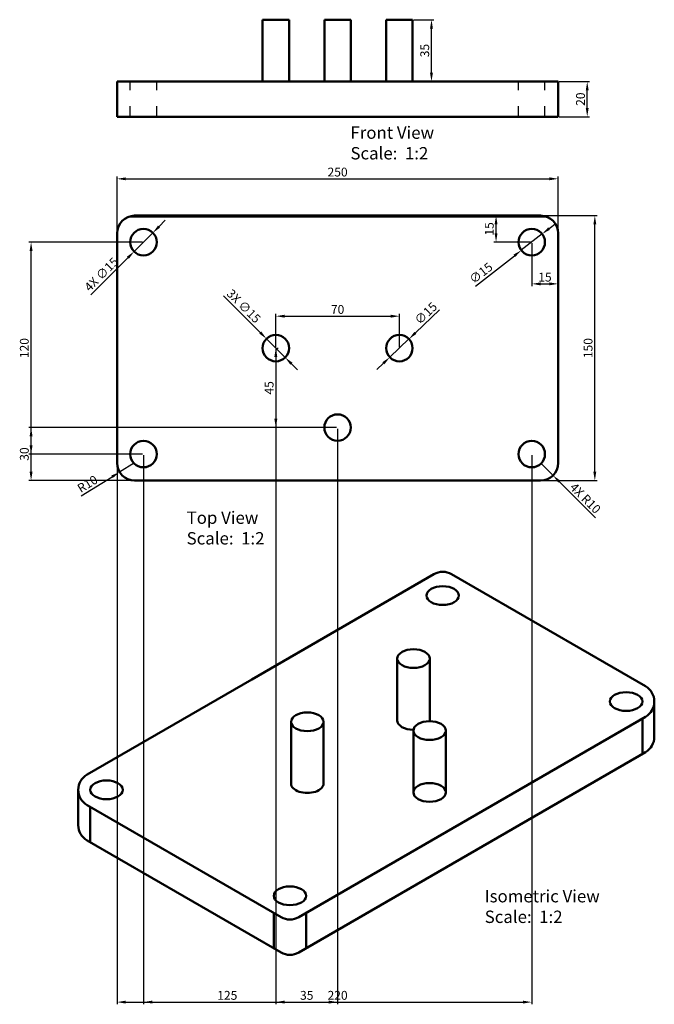
# Model space of a CAD drawing. Units: millimetres. Extents: x 2577 to 3382, y -259 to 299.
# Tile 1 of 2: x 2577 to 2937, y -259 to 299. Entities that reach past the tile are written whole.
import ezdxf

# ---------------------------------------------------------------- set-up
doc = ezdxf.new("R2010")
doc.units = ezdxf.units.MM
doc.linetypes.add('ACAD_ISO03W100', pattern=[30, 12, -18])
for name, color, linetype, lineweight in [('M-DIMS', 2, 'Continuous', 25), ('M-HIDN', 7, 'ACAD_ISO03W100', 25), ('M-OUTL', 7, 'Continuous', 50), ('M-TEXT', 7, 'Continuous', 25)]:
    doc.layers.add(name, color=color, linetype=linetype, lineweight=lineweight)
doc.styles.get("Standard").update_dxf_attribs({"font": 'arial.ttf'})
doc.dimstyles.new('ISO-25', dxfattribs={"dimtxt": 5, "dimasz": 5, "dimexe": 1.25, "dimexo": 0.625, "dimtad": 1, "dimdec": 0, "dimtxsty": 'Standard', "dimcen": 2.5, "dimadec": 0, "dimazin": 0, "dimtfac": 1, "dimtdec": 0, "dimtmove": 0, "dimatfit": 3, "dimfxl": 1, "dimarcsym": 0})

# ---------------------------------------------------------------- blocks, each defined once
blk = doc.blocks.new('*D1')
at = {"layer": 'Defpoints', "color": 0, "transparency": 16777216}
for p in [(2792.35, 130.65), (2722.35, 112.58), (2792.35, 112.58)]:
    blk.add_point(p, dxfattribs=at)
at = {"layer": 'M-DIMS', "color": 0, "lineweight": -2, "transparency": 16777216}
for p, q in [((2722.35, 113.2), (2722.35, 131.9)), ((2727.35, 130.65), (2787.35, 130.65)), ((2792.35, 113.2), (2792.35, 131.9))]:
    blk.add_line(p, q, dxfattribs=at)
at = {"layer": 'M-DIMS', "color": 0, "transparency": 16777216}
for points in [[(2727.35, 131.49), (2727.35, 129.82), (2722.35, 130.65)], [(2787.35, 131.49), (2787.35, 129.82), (2792.35, 130.65)]]:
    blk.add_solid(points, dxfattribs=at)
at = {"layer": 'M-DIMS', "color": 0, "transparency": 16777216, "insert": (2757.35, 133.83), "char_height": 5, "attachment_point": 5}
blk.add_mtext('70', dxfattribs=at)
blk = doc.blocks.new('*D2')
at = {"layer": 'Defpoints', "color": 0, "transparency": 16777216}
for p in [(2722.35, 112.58), (2722.35, 67.58), (2757.35, 67.58)]:
    blk.add_point(p, dxfattribs=at)
at = {"layer": 'M-DIMS', "color": 0, "lineweight": -2, "transparency": 16777216}
for p, q in [((2722.97, 112.58), (2723.6, 112.58)), ((2722.35, 107.58), (2722.35, 72.58)), ((2756.72, 67.58), (2721.1, 67.58))]:
    blk.add_line(p, q, dxfattribs=at)
at = {"layer": 'M-DIMS', "color": 0, "transparency": 16777216}
for points in [[(2721.52, 107.58), (2723.18, 107.58), (2722.35, 112.58)], [(2721.52, 72.58), (2723.18, 72.58), (2722.35, 67.58)]]:
    blk.add_solid(points, dxfattribs=at)
at = {"layer": 'M-DIMS', "color": 0, "transparency": 16777216, "insert": (2719.18, 90.08), "char_height": 5, "attachment_point": 5, "rotation": 90}
blk.add_mtext('45', dxfattribs=at)
blk = doc.blocks.new('*D3')
at = {"layer": 'Defpoints', "color": 0, "transparency": 16777216}
for p in [(2882.35, 208.44), (2632.35, 177.58), (2882.35, 177.58)]:
    blk.add_point(p, dxfattribs=at)
at = {"layer": 'M-DIMS', "color": 0, "lineweight": -2, "transparency": 16777216}
for p, q in [((2632.35, 178.2), (2632.35, 209.69)), ((2637.35, 208.44), (2877.35, 208.44)), ((2882.35, 178.2), (2882.35, 209.69))]:
    blk.add_line(p, q, dxfattribs=at)
at = {"layer": 'M-DIMS', "color": 0, "transparency": 16777216}
for points in [[(2637.35, 209.27), (2637.35, 207.61), (2632.35, 208.44)], [(2877.35, 209.27), (2877.35, 207.61), (2882.35, 208.44)]]:
    blk.add_solid(points, dxfattribs=at)
at = {"layer": 'M-DIMS', "color": 0, "transparency": 16777216, "insert": (2757.35, 211.62), "char_height": 5, "attachment_point": 5}
blk.add_mtext('250', dxfattribs=at)
blk = doc.blocks.new('*D4')
at = {"layer": 'Defpoints', "color": 0, "transparency": 16777216}
for p in [(2872.35, 187.58), (2903.11, 187.58), (2872.35, 37.58)]:
    blk.add_point(p, dxfattribs=at)
at = {"layer": 'M-DIMS', "color": 0, "lineweight": -2, "transparency": 16777216}
for p, q in [((2872.97, 187.58), (2904.36, 187.58)), ((2903.11, 42.58), (2903.11, 182.58)), ((2872.97, 37.58), (2904.36, 37.58))]:
    blk.add_line(p, q, dxfattribs=at)
at = {"layer": 'M-DIMS', "color": 0, "transparency": 16777216}
for points in [[(2902.28, 182.58), (2903.94, 182.58), (2903.11, 187.58)], [(2902.28, 42.58), (2903.94, 42.58), (2903.11, 37.58)]]:
    blk.add_solid(points, dxfattribs=at)
at = {"layer": 'M-DIMS', "color": 0, "transparency": 16777216, "insert": (2899.93, 112.58), "char_height": 5, "attachment_point": 5, "rotation": 90}
blk.add_mtext('150', dxfattribs=at)
blk = doc.blocks.new('*D5')
at = {"layer": 'Defpoints', "color": 0, "transparency": 16777216}
for p in [(2847.14, 187.58), (2867.35, 187.58), (2867.35, 172.58)]:
    blk.add_point(p, dxfattribs=at)
at = {"layer": 'M-DIMS', "color": 0, "lineweight": -2, "transparency": 16777216}
for p, q in [((2866.72, 187.58), (2845.89, 187.58)), ((2847.14, 177.58), (2847.14, 182.58)), ((2866.72, 172.58), (2845.89, 172.58))]:
    blk.add_line(p, q, dxfattribs=at)
at = {"layer": 'M-DIMS', "color": 0, "transparency": 16777216}
for points in [[(2846.31, 182.58), (2847.97, 182.58), (2847.14, 187.58)], [(2846.31, 177.58), (2847.97, 177.58), (2847.14, 172.58)]]:
    blk.add_solid(points, dxfattribs=at)
at = {"layer": 'M-DIMS', "color": 0, "transparency": 16777216, "insert": (2843.96, 180.08), "char_height": 5, "attachment_point": 5, "rotation": 90}
blk.add_mtext('15', dxfattribs=at)
blk = doc.blocks.new('*D6')
at = {"layer": 'Defpoints', "color": 0, "transparency": 16777216}
for p in [(2867.35, 172.58), (2882.35, 172.58), (2882.35, 148.96)]:
    blk.add_point(p, dxfattribs=at)
at = {"layer": 'M-DIMS', "color": 0, "lineweight": -2, "transparency": 16777216}
for p, q in [((2867.35, 171.95), (2867.35, 147.71)), ((2882.35, 171.95), (2882.35, 147.71)), ((2872.35, 148.96), (2877.35, 148.96))]:
    blk.add_line(p, q, dxfattribs=at)
at = {"layer": 'M-DIMS', "color": 0, "transparency": 16777216}
for points in [[(2872.35, 149.79), (2872.35, 148.12), (2867.35, 148.96)], [(2877.35, 149.79), (2877.35, 148.12), (2882.35, 148.96)]]:
    blk.add_solid(points, dxfattribs=at)
at = {"layer": 'M-DIMS', "color": 0, "transparency": 16777216, "insert": (2874.85, 152.13), "char_height": 5, "attachment_point": 5}
blk.add_mtext('15', dxfattribs=at)
blk = doc.blocks.new('*D7')
at = {"layer": 'Defpoints', "color": 0, "transparency": 16777216}
for p in [(2642.35, 47.58), (2633.82, 42.35)]:
    blk.add_point(p, dxfattribs=at)
at = {"layer": 'M-DIMS', "color": 0, "lineweight": -2, "transparency": 16777216}
for p, q in [((2642.35, 47.58), (2633.82, 42.35)), ((2612.01, 28.97), (2629.56, 39.73))]:
    blk.add_line(p, q, dxfattribs=at)
at = {"layer": 'M-DIMS', "color": 0, "transparency": 16777216}
blk.add_solid([(2629.13, 40.44), (2630, 39.02), (2633.82, 42.35)], dxfattribs=at)
at = {"layer": 'M-DIMS', "color": 0, "transparency": 16777216, "insert": (2615.96, 35.12), "char_height": 5, "attachment_point": 5, "rotation": 31.518}
blk.add_mtext('R10', dxfattribs=at)
blk = doc.blocks.new('*D8')
at = {"layer": 'Defpoints', "color": 0, "transparency": 16777216}
for p in [(2797.79, 117.74), (2786.91, 107.41)]:
    blk.add_point(p, dxfattribs=at)
at = {"layer": 'M-DIMS', "color": 0, "lineweight": -2, "transparency": 16777216}
for p, q in [((2815.1, 134.2), (2801.41, 121.19)), ((2786.91, 107.41), (2797.79, 117.74)), ((2783.29, 103.96), (2779.67, 100.52))]:
    blk.add_line(p, q, dxfattribs=at)
at = {"layer": 'M-DIMS', "color": 0, "transparency": 16777216}
for points in [[(2800.84, 121.79), (2801.98, 120.58), (2797.79, 117.74)], [(2782.72, 104.57), (2783.86, 103.36), (2786.91, 107.41)]]:
    blk.add_solid(points, dxfattribs=at)
at = {"layer": 'M-DIMS', "color": 0, "transparency": 16777216, "insert": (2807.78, 131.82), "char_height": 5, "attachment_point": 5, "rotation": 43.5491}
blk.add_mtext('∅15', dxfattribs=at)
blk = doc.blocks.new('*D9')
at = {"layer": 'Defpoints', "color": 0, "transparency": 16777216}
for p in [(2873.26, 177.2), (2861.44, 167.95)]:
    blk.add_point(p, dxfattribs=at)
at = {"layer": 'M-DIMS', "color": 0, "lineweight": -2, "transparency": 16777216}
for p, q in [((2877.19, 180.28), (2881.13, 183.36)), ((2873.26, 177.2), (2861.44, 167.95)), ((2835.55, 147.69), (2857.5, 164.87))]:
    blk.add_line(p, q, dxfattribs=at)
at = {"layer": 'M-DIMS', "color": 0, "transparency": 16777216}
for points in [[(2876.68, 180.93), (2877.71, 179.62), (2873.26, 177.2)], [(2856.99, 165.53), (2858.02, 164.22), (2861.44, 167.95)]]:
    blk.add_solid(points, dxfattribs=at)
at = {"layer": 'M-DIMS', "color": 0, "transparency": 16777216, "insert": (2838.97, 154.58), "char_height": 5, "attachment_point": 5, "rotation": 38.04}
blk.add_mtext('∅15', dxfattribs=at)
blk = doc.blocks.new('*D10')
at = {"layer": 'Defpoints', "color": 0, "transparency": 16777216}
for p in [(2799.85, 298.55), (2810.55, 298.55), (2799.85, 263.55)]:
    blk.add_point(p, dxfattribs=at)
at = {"layer": 'M-DIMS', "color": 0, "lineweight": -2, "transparency": 16777216}
for p, q in [((2800.47, 298.55), (2811.8, 298.55)), ((2810.55, 268.55), (2810.55, 293.55)), ((2800.47, 263.55), (2811.8, 263.55))]:
    blk.add_line(p, q, dxfattribs=at)
at = {"layer": 'M-DIMS', "color": 0, "transparency": 16777216}
for points in [[(2809.71, 293.55), (2811.38, 293.55), (2810.55, 298.55)], [(2809.71, 268.55), (2811.38, 268.55), (2810.55, 263.55)]]:
    blk.add_solid(points, dxfattribs=at)
at = {"layer": 'M-DIMS', "color": 0, "transparency": 16777216, "insert": (2807.37, 281.05), "char_height": 5, "attachment_point": 5, "rotation": 90}
blk.add_mtext('35', dxfattribs=at)
blk = doc.blocks.new('*D11')
at = {"layer": 'Defpoints', "color": 0, "transparency": 16777216}
for p in [(2882.35, 263.55), (2898.8, 263.55), (2882.35, 243.55)]:
    blk.add_point(p, dxfattribs=at)
at = {"layer": 'M-DIMS', "color": 0, "lineweight": -2, "transparency": 16777216}
for p, q in [((2882.97, 263.55), (2900.05, 263.55)), ((2898.8, 248.55), (2898.8, 258.55)), ((2882.97, 243.55), (2900.05, 243.55))]:
    blk.add_line(p, q, dxfattribs=at)
at = {"layer": 'M-DIMS', "color": 0, "transparency": 16777216}
for points in [[(2897.97, 258.55), (2899.63, 258.55), (2898.8, 263.55)], [(2897.97, 248.55), (2899.63, 248.55), (2898.8, 243.55)]]:
    blk.add_solid(points, dxfattribs=at)
at = {"layer": 'M-DIMS', "color": 0, "transparency": 16777216, "insert": (2895.62, 253.55), "char_height": 5, "attachment_point": 5, "rotation": 90}
blk.add_mtext('20', dxfattribs=at)
blk = doc.blocks.new('PIN-D15-H35-FRONT')
for p, q in [((-7.5, 35), (-7.5, 0)), ((7.5, 35), (-7.5, 35)), ((7.5, 35), (7.5, 0))]:
    blk.add_line(p, q)
blk = doc.blocks.new('PIN-D15-H35-ISO')
for p, q in [((-9.19, 0), (-9.19, 35)), ((9.19, 0), (9.19, 35))]:
    blk.add_line(p, q)
blk.add_ellipse((0, 35), major_axis=(-9.19, 0), ratio=0.57735)
blk = doc.blocks.new('BORE-D15-T20-FRONT')
at = {"ltscale": 0.5}
for p, q in [((-7.5, 0), (-7.5, 20)), ((7.5, 0), (7.5, 20))]:
    blk.add_line(p, q, dxfattribs=at)
blk = doc.blocks.new('BORE-D15-TOP')
blk.add_circle((0, 0), 7.5)
blk = doc.blocks.new('BORE-D15-ISO')
blk.add_ellipse((0, 0), major_axis=(-9.19, 0), ratio=0.57735)
blk = doc.blocks.new('PIN-D15-TOP')
blk.add_circle((0, 0), 7.5)
blk = doc.blocks.new('*D25')
at = {"layer": 'Defpoints', "color": 0, "transparency": 16777216}
for p in [(2757.35, 67.58), (2632.35, 47.58), (2757.35, -257.75)]:
    blk.add_point(p, dxfattribs=at)
at = {"layer": 'M-DIMS', "color": 0, "lineweight": -2, "transparency": 16777216}
for p, q in [((2757.35, 66.95), (2757.35, -259)), ((2632.35, 46.95), (2632.35, -259)), ((2637.35, -257.75), (2752.35, -257.75))]:
    blk.add_line(p, q, dxfattribs=at)
at = {"layer": 'M-DIMS', "color": 0, "transparency": 16777216}
for points in [[(2637.35, -256.92), (2637.35, -258.58), (2632.35, -257.75)], [(2752.35, -256.92), (2752.35, -258.58), (2757.35, -257.75)]]:
    blk.add_solid(points, dxfattribs=at)
at = {"layer": 'M-DIMS', "color": 0, "transparency": 16777216, "insert": (2694.85, -254.57), "char_height": 5, "attachment_point": 5}
blk.add_mtext('125', dxfattribs=at)
blk = doc.blocks.new('*D26')
at = {"layer": 'Defpoints', "color": 0, "transparency": 16777216}
for p in [(2583.66, 67.58), (2757.35, 67.58), (2642.35, 37.58)]:
    blk.add_point(p, dxfattribs=at)
at = {"layer": 'M-DIMS', "color": 0, "lineweight": -2, "transparency": 16777216}
for p, q in [((2756.72, 67.58), (2582.41, 67.58)), ((2583.66, 42.58), (2583.66, 62.58)), ((2641.72, 37.58), (2582.41, 37.58))]:
    blk.add_line(p, q, dxfattribs=at)
at = {"layer": 'M-DIMS', "color": 0, "transparency": 16777216}
for points in [[(2582.83, 62.58), (2584.5, 62.58), (2583.66, 67.58)], [(2582.83, 42.58), (2584.5, 42.58), (2583.66, 37.58)]]:
    blk.add_solid(points, dxfattribs=at)
at = {"layer": 'M-DIMS', "color": 0, "transparency": 16777216, "insert": (2580.48, 52.58), "char_height": 5, "attachment_point": 5, "rotation": 90}
blk.add_mtext('30', dxfattribs=at)
blk = doc.blocks.new('*D27')
at = {"layer": 'Defpoints', "color": 0, "transparency": 16777216}
for p in [(2722.35, 112.58), (2757.35, 67.58), (2757.35, -257.75)]:
    blk.add_point(p, dxfattribs=at)
at = {"layer": 'M-DIMS', "color": 0, "lineweight": -2, "transparency": 16777216}
for p, q in [((2722.35, 111.95), (2722.35, -259)), ((2757.35, 66.95), (2757.35, -259)), ((2727.35, -257.75), (2752.35, -257.75))]:
    blk.add_line(p, q, dxfattribs=at)
at = {"layer": 'M-DIMS', "color": 0, "transparency": 16777216}
for points in [[(2727.35, -256.92), (2727.35, -258.58), (2722.35, -257.75)], [(2752.35, -256.92), (2752.35, -258.58), (2757.35, -257.75)]]:
    blk.add_solid(points, dxfattribs=at)
at = {"layer": 'M-DIMS', "color": 0, "transparency": 16777216, "insert": (2739.85, -254.57), "char_height": 5, "attachment_point": 5}
blk.add_mtext('35', dxfattribs=at)
blk = doc.blocks.new('*D36')
at = {"layer": 'Defpoints', "color": 0, "transparency": 16777216}
for p in [(2647.35, 52.58), (2867.35, 52.58), (2867.35, -257.75)]:
    blk.add_point(p, dxfattribs=at)
at = {"layer": 'M-DIMS', "color": 0, "lineweight": -2, "transparency": 16777216}
for p, q in [((2647.35, 51.95), (2647.35, -259)), ((2867.35, 51.95), (2867.35, -259)), ((2652.35, -257.75), (2862.35, -257.75))]:
    blk.add_line(p, q, dxfattribs=at)
at = {"layer": 'M-DIMS', "color": 0, "transparency": 16777216}
for points in [[(2652.35, -256.92), (2652.35, -258.58), (2647.35, -257.75)], [(2862.35, -256.92), (2862.35, -258.58), (2867.35, -257.75)]]:
    blk.add_solid(points, dxfattribs=at)
at = {"layer": 'M-DIMS', "color": 0, "transparency": 16777216, "insert": (2757.35, -254.57), "char_height": 5, "attachment_point": 5}
blk.add_mtext('220', dxfattribs=at)
blk = doc.blocks.new('*D37')
at = {"layer": 'Defpoints', "color": 0, "transparency": 16777216}
for p in [(2583.66, 172.58), (2647.35, 172.58), (2647.35, 52.58)]:
    blk.add_point(p, dxfattribs=at)
at = {"layer": 'M-DIMS', "color": 0, "lineweight": -2, "transparency": 16777216}
for p, q in [((2646.72, 172.58), (2582.41, 172.58)), ((2583.66, 57.58), (2583.66, 167.58)), ((2646.72, 52.58), (2582.41, 52.58))]:
    blk.add_line(p, q, dxfattribs=at)
at = {"layer": 'M-DIMS', "color": 0, "transparency": 16777216}
for points in [[(2582.83, 167.58), (2584.5, 167.58), (2583.66, 172.58)], [(2582.83, 57.58), (2584.5, 57.58), (2583.66, 52.58)]]:
    blk.add_solid(points, dxfattribs=at)
at = {"layer": 'M-DIMS', "color": 0, "transparency": 16777216, "insert": (2580.48, 112.58), "char_height": 5, "attachment_point": 5, "rotation": 90}
blk.add_mtext('120', dxfattribs=at)
blk = doc.blocks.new('*D38')
at = {"layer": 'Defpoints', "color": 0, "transparency": 16777216}
for p in [(2717.05, 117.88), (2727.65, 107.27)]:
    blk.add_point(p, dxfattribs=at)
at = {"layer": 'M-DIMS', "color": 0, "lineweight": -2, "transparency": 16777216}
for p, q in [((2692.76, 142.19), (2713.51, 121.42)), ((2727.65, 107.27), (2717.05, 117.88)), ((2731.18, 103.73), (2734.72, 100.2))]:
    blk.add_line(p, q, dxfattribs=at)
at = {"layer": 'M-DIMS', "color": 0, "transparency": 16777216}
for points in [[(2714.1, 122.01), (2712.93, 120.83), (2717.05, 117.88)], [(2731.77, 104.32), (2730.59, 103.14), (2727.65, 107.27)]]:
    blk.add_solid(points, dxfattribs=at)
at = {"layer": 'M-DIMS', "color": 0, "transparency": 16777216, "insert": (2703.72, 135.92), "char_height": 5, "attachment_point": 5, "rotation": 314.9742}
blk.add_mtext('3X ∅15', dxfattribs=at)
blk = doc.blocks.new('*D39')
at = {"layer": 'Defpoints', "color": 0, "transparency": 16777216}
for p in [(2872.35, 47.58), (2879.42, 40.5)]:
    blk.add_point(p, dxfattribs=at)
at = {"layer": 'M-DIMS', "color": 0, "lineweight": -2, "transparency": 16777216}
for p, q in [((2872.35, 47.58), (2879.42, 40.5)), ((2903.55, 16.38), (2882.96, 36.97))]:
    blk.add_line(p, q, dxfattribs=at)
at = {"layer": 'M-DIMS', "color": 0, "transparency": 16777216}
blk.add_solid([(2883.55, 37.56), (2882.37, 36.38), (2879.42, 40.5)], dxfattribs=at)
at = {"layer": 'M-DIMS', "color": 0, "transparency": 16777216, "insert": (2897.27, 27.15), "char_height": 5, "attachment_point": 5, "rotation": 315.0032}
blk.add_mtext('4X R10', dxfattribs=at)
blk = doc.blocks.new('*D40')
at = {"layer": 'Defpoints', "color": 0, "transparency": 16777216}
for p in [(2652.65, 177.88), (2642.04, 167.27)]:
    blk.add_point(p, dxfattribs=at)
at = {"layer": 'M-DIMS', "color": 0, "lineweight": -2, "transparency": 16777216}
for p, q in [((2656.19, 181.41), (2659.73, 184.95)), ((2652.65, 177.88), (2642.04, 167.27)), ((2617.59, 142.84), (2638.51, 163.74))]:
    blk.add_line(p, q, dxfattribs=at)
at = {"layer": 'M-DIMS', "color": 0, "transparency": 16777216}
for points in [[(2655.6, 182), (2656.78, 180.82), (2652.65, 177.88)], [(2637.92, 164.33), (2639.1, 163.15), (2642.04, 167.27)]]:
    blk.add_solid(points, dxfattribs=at)
at = {"layer": 'M-DIMS', "color": 0, "transparency": 16777216, "insert": (2623.94, 153.87), "char_height": 5, "attachment_point": 5, "rotation": 44.9783}
blk.add_mtext('4X ∅15', dxfattribs=at)

msp = doc.modelspace()

# ---------------------------------------------------------------- linework, layer by layer
at = {"layer": 'M-OUTL'}
for p, q in [((2784.85, 298.55), (2784.85, 263.55)), ((2799.85, 298.55), (2799.85, 263.55)), ((2882.35, 263.55), (2632.35, 263.55)), ((2632.35, 263.55), (2632.35, 243.55)), ((2882.35, 243.55), (2882.35, 263.55)), ((2632.35, 243.55), (2882.35, 243.55)), ((2875.11, 187.19), (2639.59, 187.19)), ((2872.35, 187.58), (2642.35, 187.58)), ((2632.35, 177.58), (2632.35, 47.58)), ((2882.35, 47.58), (2882.35, 177.58)), ((2642.35, 37.58), (2872.35, 37.58)), ((2708.67, -75.05), (2811.92, -15.43)), ((2821.92, -15.43), (2931.82, -78.89)), ((2708.67, -75.05), (2615.41, -128.89)), ((2936.82, -87.55), (2936.82, -107.55)), ((2931.82, -96.21), (2735.32, -209.66)), ((2930.03, -97.24), (2930.03, -117.24)), ((2735.32, -229.66), (2931.82, -116.21)), ((2610.41, -137.55), (2610.41, -157.55)), ((2725.32, -209.66), (2615.41, -146.21)), ((2617.21, -147.24), (2617.21, -167.24)), ((2615.41, -166.21), (2725.32, -229.66)), ((2721.13, -207.24), (2721.13, -227.24)), ((2739.5, -207.24), (2739.5, -227.24))]:
    msp.add_line(p, q, dxfattribs=at)
for centre, start, end in [((2642.35, 177.58), 90, 180), ((2872.35, 177.58), 0, 90), ((2642.35, 47.58), 180, 270), ((2872.35, 47.58), 270, 0), ((2816.92, -24.09), 60, 120), ((2926.82, -87.55), 300, 60), ((2926.82, -107.55), 300, 0), ((2620.41, -137.55), 120, 240), ((2620.41, -157.55), 180, 240), ((2730.32, -201), 240, 300), ((2730.32, -221), 240, 300)]:
    msp.add_arc(centre, 10, start, end, dxfattribs=at)
for centre, start_param, end_param in [((2800.35, -98.25), 0, 1.566742), ((2800.35, -98.25), 3.054795, 3.141593), ((2740.18, -134.02), 0, 3.141593)]:
    msp.add_ellipse(centre, major_axis=(-9.19, 0), ratio=0.57735, start_param=start_param, end_param=end_param, dxfattribs=at)
msp.add_ellipse((2809.46, -139.02), major_axis=(-9.19, 0), ratio=0.57735, dxfattribs=at)

# ---------------------------------------------------------------- block references
at = {"layer": 'M-HIDN'}
for p in [(2647.35, 243.55), (2867.35, 243.55)]:
    msp.add_blockref('BORE-D15-T20-FRONT', p, dxfattribs=at)
at = {"layer": 'M-OUTL'}
for name, p in [('PIN-D15-H35-FRONT', (2722.35, 263.55)), ('PIN-D15-H35-FRONT', (2757.35, 263.55)), ('PIN-D15-H35-FRONT', (2792.35, 263.55)), ('BORE-D15-TOP', (2647.35, 172.58)), ('BORE-D15-TOP', (2867.35, 172.58)), ('PIN-D15-TOP', (2722.35, 112.58)), ('PIN-D15-TOP', (2792.35, 112.58)), ('PIN-D15-TOP', (2757.35, 67.58)), ('BORE-D15-TOP', (2647.35, 52.58)), ('BORE-D15-TOP', (2867.35, 52.58)), ('BORE-D15-ISO', (2816.92, -27.55)), ('PIN-D15-H35-ISO', (2800.35, -98.25)), ('BORE-D15-ISO', (2920.84, -87.55)), ('PIN-D15-H35-ISO', (2740.18, -134.02)), ('PIN-D15-H35-ISO', (2809.46, -139.02)), ('BORE-D15-ISO', (2626.39, -137.55)), ('BORE-D15-ISO', (2730.32, -197.55))]:
    msp.add_blockref(name, p, dxfattribs=at)

# ---------------------------------------------------------------- texts
at = {"layer": 'M-TEXT', "char_height": 7, "attachment_point": 1}
for s, insert in [('Front View\\PScale:  1:2', (2764.63, 238.09)), ('Top View\\PScale:  1:2', (2671.8, 20.05)), ('Isometric View\\PScale:  1:2', (2840.71, -194.28))]:
    msp.add_mtext_dynamic_manual_height_columns(s, width=128.7125, gutter_width=12.5, heights=[0], dxfattribs=dict(at, insert=insert))

# ---------------------------------------------------------------- dimensions: what is measured, and where the dimension line sits
at = {"layer": 'M-DIMS'}
for base, p1, p2, override, picture, middle in [((2810.55, 298.55), (2799.85, 263.55), (2799.85, 298.55), {"dimclrd": 0, "dimclre": 0, "dimclrt": 0}, '*D10', (2807.37, 281.05)), ((2898.8, 263.55), (2882.35, 243.55), (2882.35, 263.55), {"dimclrd": 0, "dimclre": 0, "dimclrt": 0}, '*D11', (2895.62, 253.55)), ((2847.14, 187.58), (2867.35, 172.58), (2867.35, 187.58), {"dimclrd": 0, "dimclre": 0, "dimclrt": 0}, '*D5', (2843.96, 180.08)), ((2903.11, 187.58), (2872.35, 37.58), (2872.35, 187.58), {"dimclrd": 0, "dimclre": 0, "dimclrt": 0}, '*D4', (2899.93, 112.58)), ((2583.66, 172.58), (2647.35, 52.58), (2647.35, 172.58), {"dimdec": 0, "dimlfac": 1, "dimrnd": 0, "dimzin": 0, "dimdsep": 46, "dimlunit": 2}, '*D37', (2580.48, 112.58)), ((2722.35, 67.58), (2722.35, 112.58), (2757.35, 67.58), {"dimclrd": 0, "dimclre": 0, "dimclrt": 0}, '*D2', (2719.18, 90.08)), ((2583.66, 67.58), (2642.35, 37.58), (2757.35, 67.58), {"dimdec": 0, "dimlfac": 1, "dimrnd": 0, "dimzin": 0, "dimdsep": 46, "dimlunit": 2}, '*D26', (2580.48, 52.58))]:
    dim = msp.add_linear_dim(base=base, p1=p1, p2=p2, angle=90, dimstyle='ISO-25', override=override, dxfattribs=at)
    dim.commit()
    dim.dimension.update_dxf_attribs({"geometry": picture, "text_midpoint": middle})
for base, p1, p2, override, picture, middle in [((2882.35, 208.44), (2632.35, 177.58), (2882.35, 177.58), {"dimclrd": 0, "dimclre": 0, "dimclrt": 0}, '*D3', (2757.35, 211.62)), ((2882.35, 148.96), (2867.35, 172.58), (2882.35, 172.58), {"dimclrd": 0, "dimclre": 0, "dimclrt": 0}, '*D6', (2874.85, 152.13)), ((2792.35, 130.65), (2722.35, 112.58), (2792.35, 112.58), {"dimclrd": 0, "dimclre": 0, "dimclrt": 0}, '*D1', (2757.35, 133.83)), ((2757.35, -257.75), (2722.35, 112.58), (2757.35, 67.58), {"dimdec": 0, "dimlfac": 1, "dimrnd": 0, "dimzin": 0, "dimdsep": 46, "dimlunit": 2}, '*D27', (2739.85, -254.57)), ((2757.35, -257.75), (2632.35, 47.58), (2757.35, 67.58), {"dimdec": 0, "dimlfac": 1, "dimrnd": 0, "dimzin": 0, "dimdsep": 46, "dimlunit": 2}, '*D25', (2694.85, -254.57)), ((2867.35, -257.75), (2647.35, 52.58), (2867.35, 52.58), {"dimdec": 0, "dimlfac": 1, "dimrnd": 0, "dimzin": 0, "dimdsep": 46, "dimlunit": 2}, '*D36', (2757.35, -254.57))]:
    dim = msp.add_linear_dim(base=base, p1=p1, p2=p2, dimstyle='ISO-25', override=override, dxfattribs=at)
    dim.commit()
    dim.dimension.update_dxf_attribs({"geometry": picture, "text_midpoint": middle})
for p1, p2, text, picture, middle in [((2652.65, 177.88), (2642.04, 167.27), '4X <>', '*D40', (2626.28, 151.52)), ((2727.65, 107.27), (2717.05, 117.88), '3X <>', '*D38', (2701.37, 133.57))]:
    dim = msp.add_diameter_dim_2p(p1=p1, p2=p2, text=text, dimstyle='ISO-25', override={"dimdec": 0, "dimlfac": 1, "dimrnd": 0, "dimzin": 0, "dimdsep": 46, "dimlunit": 2}, dxfattribs=at)
    dim.commit()
    dim.dimension.update_dxf_attribs({"geometry": picture, "text_midpoint": middle, "dimtype": 163})
dim = msp.add_diameter_dim_2p(p1=(2873.26, 177.2), p2=(2861.44, 167.95), dimstyle='ISO-25', override={"dimclrd": 0, "dimclre": 0, "dimclrt": 0}, dxfattribs=at)
dim.commit()
dim.dimension.update_dxf_attribs({"geometry": '*D9', "text_midpoint": (2841.01, 151.97), "dimtype": 163})
dim = msp.add_diameter_dim_2p(p1=(2786.91, 107.41), p2=(2797.79, 117.74), dimstyle='ISO-25', override={"dimclrd": 0, "dimclre": 0, "dimclrt": 0}, dxfattribs=at)
dim.commit()
dim.dimension.update_dxf_attribs({"geometry": '*D8', "text_midpoint": (2807.78, 131.82)})
dim = msp.add_radius_dim(center=(2642.35, 47.58), mpoint=(2633.82, 42.35), dimstyle='ISO-25', override={"dimclrd": 0, "dimclre": 0, "dimclrt": 0}, dxfattribs=at)
dim.commit()
dim.dimension.update_dxf_attribs({"geometry": '*D7', "text_midpoint": (2617.62, 32.41), "dimtype": 164})
dim = msp.add_radius_dim(center=(2872.35, 47.58), mpoint=(2879.42, 40.5), text='4X <>', dimstyle='ISO-25', override={"dimdec": 0, "dimlfac": 1, "dimrnd": 0, "dimzin": 0, "dimdsep": 46, "dimlunit": 2}, dxfattribs=at)
dim.commit()
dim.dimension.update_dxf_attribs({"geometry": '*D39', "text_midpoint": (2897.27, 27.15)})

doc.saveas('drawing.dxf')
